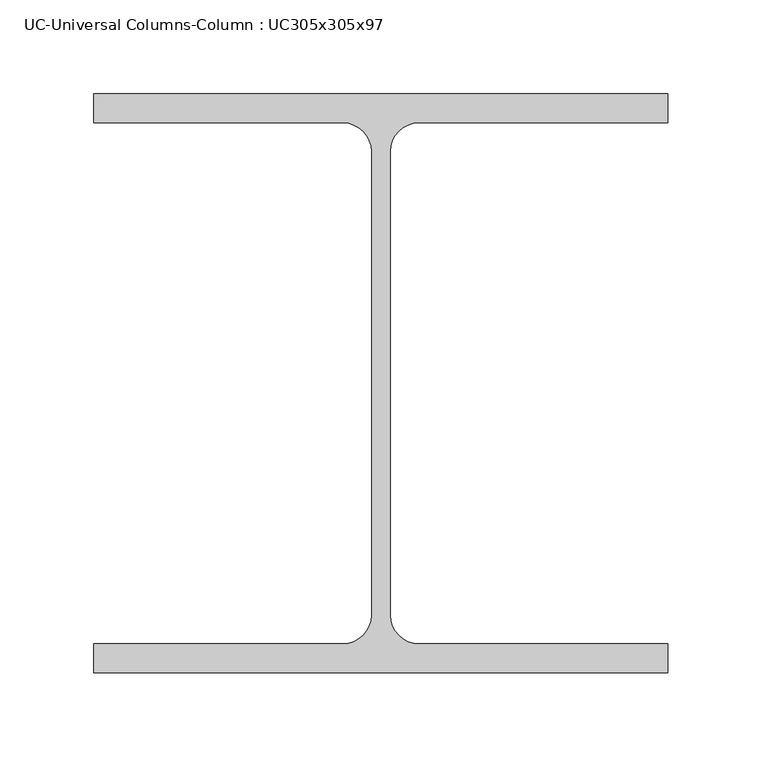
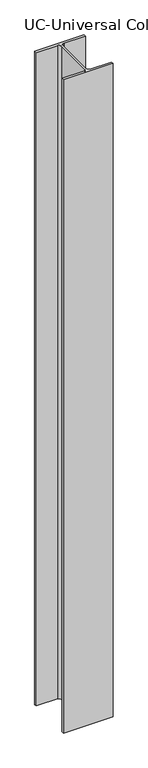
"""IFC4 building model written with IfcOpenShell, lengths in millimetres: column geometry, UC-Universal Columns-Column : UC305x305x97."""

from ifc_helpers import new_model, si_unit, point, frame_2d, origin, origin_with_axes, place, context, project, spatial, polyline, circle_curve, trimmed, segment, composite_curve, outline, extrude, source, transform, mapped, element, save


def uc_universal_columns_column_uc305x305x97_11a20181(model_context):
    return source(origin(), model_context, "Body", "SweptSolid", [
        extrude(outline(composite_curve([segment(polyline([(152.65, 153.95), (152.65, 138.55), (20.15, 138.55)]), True, "CONTINUOUS"), segment(trimmed(circle_curve(frame_2d((20.15, 123.35)), 15.2), [point((20.15, 138.55))], [point((4.95, 123.35))], True, "CARTESIAN"), True, "CONTINUOUS"), segment(polyline([(4.95, 123.35), (4.95, -123.35)]), True, "CONTINUOUS"), segment(trimmed(circle_curve(frame_2d((20.15, -123.35)), 15.2), [point((4.95, -123.35))], [point((20.15, -138.55))], True, "CARTESIAN"), True, "CONTINUOUS"), segment(polyline([(20.15, -138.55), (152.65, -138.55), (152.65, -153.95), (-152.65, -153.95), (-152.65, -138.55), (-20.15, -138.55)]), True, "CONTINUOUS"), segment(trimmed(circle_curve(frame_2d((-20.15, -123.35)), 15.2), [point((-20.15, -138.55))], [point((-4.95, -123.35))], True, "CARTESIAN"), True, "CONTINUOUS"), segment(polyline([(-4.95, -123.35), (-4.95, 123.35)]), True, "CONTINUOUS"), segment(trimmed(circle_curve(frame_2d((-20.15, 123.35)), 15.2), [point((-4.95, 123.35))], [point((-20.15, 138.55))], True, "CARTESIAN"), True, "CONTINUOUS"), segment(polyline([(-20.15, 138.55), (-152.65, 138.55), (-152.65, 153.95), (152.65, 153.95)]), True, "CONTINUOUS")], self_intersect=False)), origin_with_axes(), (0.0, 0.0, 1.0), 4267.0),
    ])


if __name__ == "__main__":
    model = new_model("IFC4")
    model_context = context("Model", 3, world=origin())
    ifc_project = project(units=[si_unit("LENGTHUNIT", "METRE", prefix="MILLI")], contexts=[model_context])
    site = spatial("IfcSite", under=ifc_project)
    building = spatial("IfcBuilding", under=site)
    placement = place(None, origin())
    uc_universal_columns_column_uc305x305x97_shape = uc_universal_columns_column_uc305x305x97_11a20181(model_context)
    element("IfcColumn", 1, ObjectType="UC-Universal Columns-Column : UC305x305x97", at=placement, inside=building, context=model_context, shape_type="MappedRepresentation", body=[
        mapped(uc_universal_columns_column_uc305x305x97_shape, transform((0.0, 0.0, 0.0), x_axis=(1.0, 0.0, 0.0), y_axis=(0.0, 1.0, 0.0), z_axis=(0.0, 0.0, 1.0))),
    ])
    save(model, "model.ifc")

# Revit data of these elements
# Type "UC-Universal Columns-Column : UC305x305x97"
#   Section Name Key = "UC305x305x97"
#   Width = 30.53 cm
#   Web Thickness = 0.99 cm
#   Web Fillet = 1.52 cm
#   Warping Constant = 1560000.0 cm⁶
#   Torsional Moment of Inertia = 91.20 cm⁴
#   Section Area = 123.0 cm²
#   Plastic Modulus weak axis = 726.0 cm³
#   Plastic Modulus strong axis = 1592.0 cm³
#   Nominal Weight = 96.8996 kgf/m
#   Moment of Inertia weak axis = 7308.00 cm⁴
#   Moment of Inertia strong axis = 22249.00 cm⁴
#   Height = 30.79 cm
#   Flange Thickness = 1.54 cm
#   Elastic Modulus weak axis = 479.0 cm³
#   Elastic Modulus strong axis = 1445.0 cm³
#   Centroid Vertical = 15.395 cm
#   Centroid Horizontal = 15.265 cm
#   Bolt Spacing = 14.0 cm
#   Structural Material [instance default] = Metal - Steel 43-275
#   Type Comments = ""
#   Assembly Code = ""
# Element 1 (IfcColumn, "UC-Universal Columns-Column : UC305x305x97")
#   Materials on its faces: "Metal - Steel 43-275"
# Materials
#   "Metal - Steel 43-275": class "Metal", colour RGB 247 247 247, transparency 0, Cost = 0
